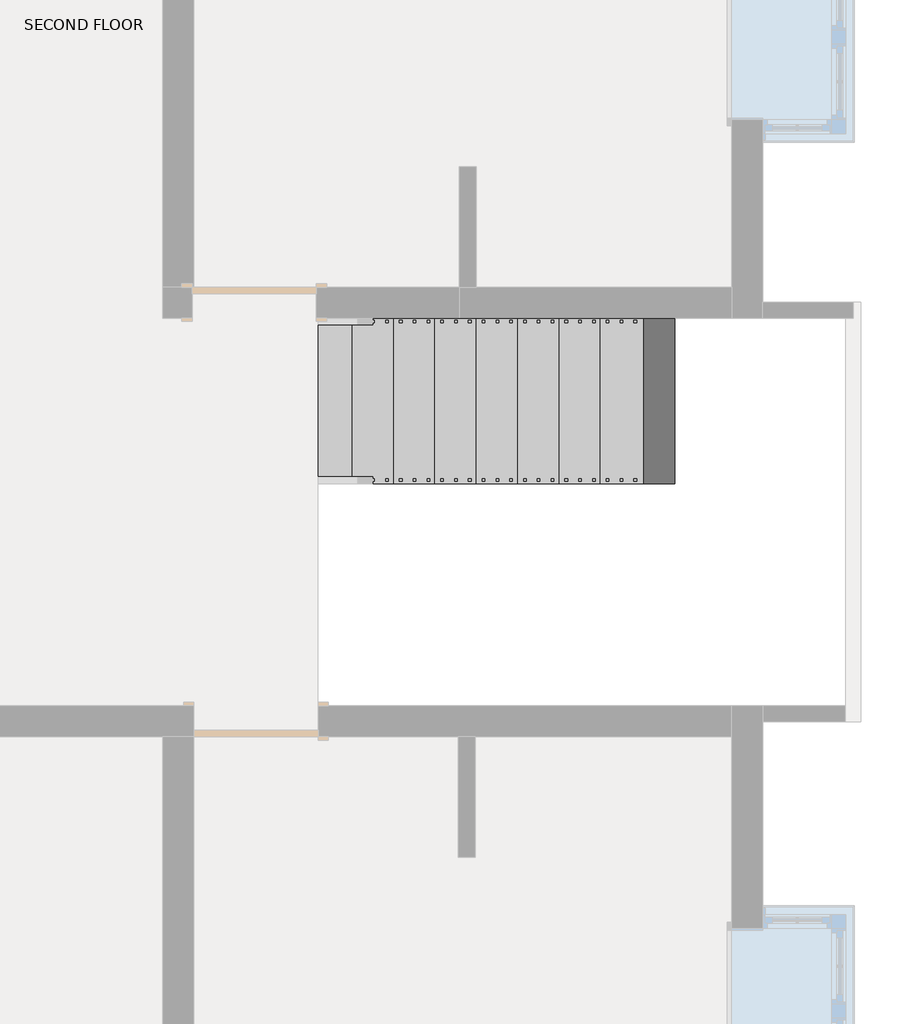
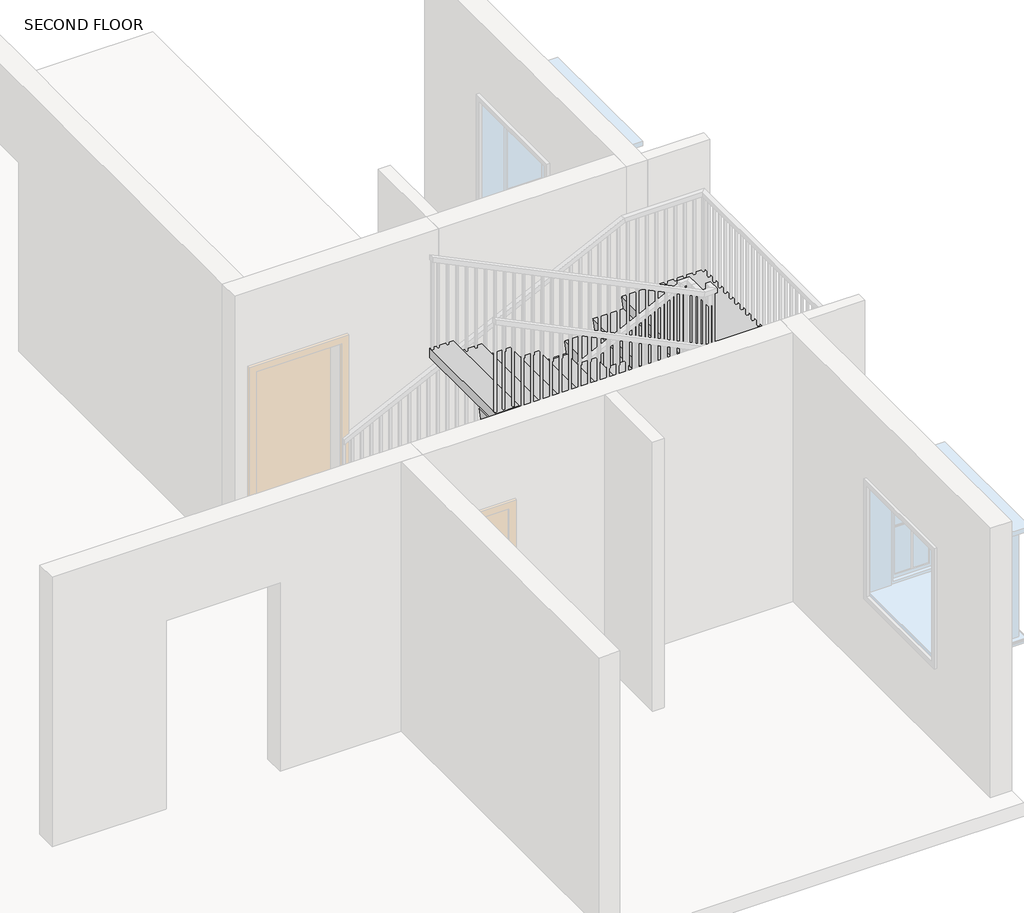
# One storey, part 3 of 6: 1 railing, 1 stair flight.
"""IFC4 building model written with IfcOpenShell, lengths in millimetres."""

from ifc_helpers import new_model, si_unit, frame, origin, place, context, project, spatial, polyline, outline, extrude, faceted_brep, element, save

model = new_model("IFC4")

# Units and contexts
model_context = context("Model", 3, world=origin())
ifc_project = project(units=[si_unit("LENGTHUNIT", "METRE", prefix="MILLI")], contexts=[model_context])

# Site, building, storey
site = spatial("IfcSite", under=ifc_project)
building = spatial("IfcBuilding", under=site)
storey = spatial("IfcBuildingStorey", under=building, Name="SECOND FLOOR", Elevation=6400.8)

# Railing
placement = place(None, origin())
element("IfcRailing", 1, ObjectType="Handrail - Rectangular", at=placement, inside=storey, context=model_context, shape_type="SolidModel", body=[
    faceted_brep([(3126.2584916, -947.666654, 7460.6727273), (3126.2584916, -947.666654, 7404.1956113), (3126.2584916, -998.466654, 7404.1956113), (3126.2584916, -998.466654, 7460.6727273), (6044.5829507, -947.666654, 8878.3823634), (6095.3829507, -947.666654, 8846.5836718), (6095.3829507, -998.466654, 8846.5836718), (6044.5829507, -998.466654, 8878.3823634), (6044.5829507, -947.666654, 8915.4), (6095.3829507, -947.666654, 8864.6), (6095.3829507, -998.466654, 8864.6), (6044.5829507, -998.466654, 8915.4), (6171.5829507, -947.666654, 8915.4), (6171.5829507, -947.666654, 8864.6), (6120.7829507, -998.466654, 8864.6), (6120.7829507, -998.466654, 8915.4), (6171.5829507, -1074.666654, 8915.4), (6171.5829507, -1074.666654, 8864.6), (6120.7829507, -1074.666654, 8864.6), (6120.7829507, -1074.666654, 8915.4), (6171.5829507, -1341.366654, 8915.4), (6171.5829507, -1392.166654, 8864.6), (6120.7829507, -1392.166654, 8864.6), (6120.7829507, -1341.366654, 8915.4), (6171.5829507, -1341.366654, 9097.8903639), (6171.5829507, -1392.166654, 9047.0903639), (6120.7829507, -1392.166654, 9047.0903639), (6120.7829507, -1341.366654, 9097.8903639), (6171.5829507, -1468.366654, 9097.8903639), (6171.5829507, -1468.366654, 9047.0903639), (6120.7829507, -1417.566654, 9047.0903639), (6120.7829507, -1417.566654, 9097.8903639), (6044.5829507, -1468.366654, 9097.8903639), (6032.8967309, -1468.366654, 9047.0903639), (6032.8967309, -1417.566654, 9047.0903639), (6044.5829507, -1417.566654, 9097.8903639), (3126.2584916, -1468.366654, 10515.6), (3126.2584916, -1417.566654, 10515.6), (3126.2584916, -1417.566654, 10459.122884), (3126.2584916, -1468.366654, 10459.122884)], [[[0, 1, 2, 3]], [[1, 0, 4, 5]], [[2, 1, 5, 6]], [[3, 2, 6, 7]], [[0, 3, 7, 4]], [[5, 4, 8, 9]], [[6, 5, 9, 10]], [[7, 6, 10, 11]], [[4, 7, 11, 8]], [[9, 8, 12, 13]], [[10, 9, 13, 14]], [[11, 10, 14, 15]], [[8, 11, 15, 12]], [[13, 12, 16, 17]], [[14, 13, 17, 18]], [[15, 14, 18, 19]], [[12, 15, 19, 16]], [[17, 16, 20, 21]], [[18, 17, 21, 22]], [[19, 18, 22, 23]], [[16, 19, 23, 20]], [[21, 20, 24, 25]], [[22, 21, 25, 26]], [[23, 22, 26, 27]], [[20, 23, 27, 24]], [[25, 24, 28, 29]], [[26, 25, 29, 30]], [[27, 26, 30, 31]], [[24, 27, 31, 28]], [[29, 28, 32, 33]], [[30, 29, 33, 34]], [[31, 30, 34, 35]], [[28, 31, 35, 32]], [[36, 37, 38, 39]], [[33, 32, 36, 39]], [[34, 33, 39, 38]], [[35, 34, 38, 37]], [[32, 35, 37, 36]]]),
    extrude(outline(polyline([(10418.7778093, 3209.3079507), (10428.0322184, 3190.2579507), (9455.7272727, 3190.2579507), (9455.7272727, 3209.3079507), (10418.7778093, 3209.3079507)])), frame((0.0, -1452.491654, 0.0), z_axis=(0.0, 1.0, 0.0), x_axis=(0.0, 0.0, 1.0)), (0.0, 0.0, 1.0), 19.05),
    extrude(outline(polyline([(10369.4209605, 3310.9079507), (10378.6753696, 3291.8579507), (9455.7272727, 3291.8579507), (9455.7272727, 3310.9079507), (10369.4209605, 3310.9079507)])), frame((0.0, -1452.491654, 0.0), z_axis=(0.0, 1.0, 0.0), x_axis=(0.0, 0.0, 1.0)), (0.0, 0.0, 1.0), 19.05),
    extrude(outline(polyline([(10320.0641117, 3412.5079507), (10329.3185208, 3393.4579507), (9310.2545455, 3393.4579507), (9310.2545455, 3412.5079507), (10320.0641117, 3412.5079507)])), frame((0.0, -1452.491654, 0.0), z_axis=(0.0, 1.0, 0.0), x_axis=(0.0, 0.0, 1.0)), (0.0, 0.0, 1.0), 19.05),
    extrude(outline(polyline([(10270.7072629, 3514.1079507), (10279.9616721, 3495.0579507), (9310.2545455, 3495.0579507), (9310.2545455, 3514.1079507), (10270.7072629, 3514.1079507)])), frame((0.0, -1452.491654, 0.0), z_axis=(0.0, 1.0, 0.0), x_axis=(0.0, 0.0, 1.0)), (0.0, 0.0, 1.0), 19.05),
    extrude(outline(polyline([(10221.3504141, 3615.7079507), (10230.6048233, 3596.6579507), (9310.2545455, 3596.6579507), (9310.2545455, 3615.7079507), (10221.3504141, 3615.7079507)])), frame((0.0, -1452.491654, 0.0), z_axis=(0.0, 1.0, 0.0), x_axis=(0.0, 0.0, 1.0)), (0.0, 0.0, 1.0), 19.05),
    extrude(outline(polyline([(10171.9935653, 3717.3079507), (10181.2479745, 3698.2579507), (9164.7818182, 3698.2579507), (9164.7818182, 3717.3079507), (10171.9935653, 3717.3079507)])), frame((0.0, -1452.491654, 0.0), z_axis=(0.0, 1.0, 0.0), x_axis=(0.0, 0.0, 1.0)), (0.0, 0.0, 1.0), 19.05),
    extrude(outline(polyline([(10122.6367166, 3818.9079507), (10131.8911257, 3799.8579507), (9164.7818182, 3799.8579507), (9164.7818182, 3818.9079507), (10122.6367166, 3818.9079507)])), frame((0.0, -1452.491654, 0.0), z_axis=(0.0, 1.0, 0.0), x_axis=(0.0, 0.0, 1.0)), (0.0, 0.0, 1.0), 19.05),
    extrude(outline(polyline([(10073.2798678, 3920.5079507), (10082.5342769, 3901.4579507), (9164.7818182, 3901.4579507), (9164.7818182, 3920.5079507), (10073.2798678, 3920.5079507)])), frame((0.0, -1452.491654, 0.0), z_axis=(0.0, 1.0, 0.0), x_axis=(0.0, 0.0, 1.0)), (0.0, 0.0, 1.0), 19.05),
    extrude(outline(polyline([(10023.923019, 4022.1079507), (10033.1774281, 4003.0579507), (9019.3090909, 4003.0579507), (9019.3090909, 4022.1079507), (10023.923019, 4022.1079507)])), frame((0.0, -1452.491654, 0.0), z_axis=(0.0, 1.0, 0.0), x_axis=(0.0, 0.0, 1.0)), (0.0, 0.0, 1.0), 19.05),
    extrude(outline(polyline([(9974.5661702, 4123.7079507), (9983.8205793, 4104.6579507), (9019.3090909, 4104.6579507), (9019.3090909, 4123.7079507), (9974.5661702, 4123.7079507)])), frame((0.0, -1452.491654, 0.0), z_axis=(0.0, 1.0, 0.0), x_axis=(0.0, 0.0, 1.0)), (0.0, 0.0, 1.0), 19.05),
    extrude(outline(polyline([(9925.2093214, 4225.3079507), (9934.4637306, 4206.2579507), (9019.3090909, 4206.2579507), (9019.3090909, 4225.3079507), (9925.2093214, 4225.3079507)])), frame((0.0, -1452.491654, 0.0), z_axis=(0.0, 1.0, 0.0), x_axis=(0.0, 0.0, 1.0)), (0.0, 0.0, 1.0), 19.05),
    extrude(outline(polyline([(9875.8524726, 4326.9079507), (9885.1068818, 4307.8579507), (8873.8363636, 4307.8579507), (8873.8363636, 4326.9079507), (9875.8524726, 4326.9079507)])), frame((0.0, -1452.491654, 0.0), z_axis=(0.0, 1.0, 0.0), x_axis=(0.0, 0.0, 1.0)), (0.0, 0.0, 1.0), 19.05),
    extrude(outline(polyline([(9826.4956238, 4428.5079507), (9835.750033, 4409.4579507), (8873.8363636, 4409.4579507), (8873.8363636, 4428.5079507), (9826.4956238, 4428.5079507)])), frame((0.0, -1452.491654, 0.0), z_axis=(0.0, 1.0, 0.0), x_axis=(0.0, 0.0, 1.0)), (0.0, 0.0, 1.0), 19.05),
    extrude(outline(polyline([(9777.1387751, 4530.1079507), (9786.3931842, 4511.0579507), (8873.8363636, 4511.0579507), (8873.8363636, 4530.1079507), (9777.1387751, 4530.1079507)])), frame((0.0, -1452.491654, 0.0), z_axis=(0.0, 1.0, 0.0), x_axis=(0.0, 0.0, 1.0)), (0.0, 0.0, 1.0), 19.05),
    extrude(outline(polyline([(9727.7819263, 4631.7079507), (9737.0363354, 4612.6579507), (8728.3636364, 4612.6579507), (8728.3636364, 4631.7079507), (9727.7819263, 4631.7079507)])), frame((0.0, -1452.491654, 0.0), z_axis=(0.0, 1.0, 0.0), x_axis=(0.0, 0.0, 1.0)), (0.0, 0.0, 1.0), 19.05),
    extrude(outline(polyline([(9678.4250775, 4733.3079507), (9687.6794866, 4714.2579507), (8728.3636364, 4714.2579507), (8728.3636364, 4733.3079507), (9678.4250775, 4733.3079507)])), frame((0.0, -1452.491654, 0.0), z_axis=(0.0, 1.0, 0.0), x_axis=(0.0, 0.0, 1.0)), (0.0, 0.0, 1.0), 19.05),
    extrude(outline(polyline([(9629.0682287, 4834.9079507), (9638.3226379, 4815.8579507), (8728.3636364, 4815.8579507), (8728.3636364, 4834.9079507), (9629.0682287, 4834.9079507)])), frame((0.0, -1452.491654, 0.0), z_axis=(0.0, 1.0, 0.0), x_axis=(0.0, 0.0, 1.0)), (0.0, 0.0, 1.0), 19.05),
    extrude(outline(polyline([(9579.7113799, 4936.5079507), (9588.9657891, 4917.4579507), (8582.8909091, 4917.4579507), (8582.8909091, 4936.5079507), (9579.7113799, 4936.5079507)])), frame((0.0, -1452.491654, 0.0), z_axis=(0.0, 1.0, 0.0), x_axis=(0.0, 0.0, 1.0)), (0.0, 0.0, 1.0), 19.05),
    extrude(outline(polyline([(9530.3545311, 5038.1079507), (9539.6089403, 5019.0579507), (8582.8909091, 5019.0579507), (8582.8909091, 5038.1079507), (9530.3545311, 5038.1079507)])), frame((0.0, -1452.491654, 0.0), z_axis=(0.0, 1.0, 0.0), x_axis=(0.0, 0.0, 1.0)), (0.0, 0.0, 1.0), 19.05),
    extrude(outline(polyline([(9480.9976824, 5139.7079507), (9490.2520915, 5120.6579507), (8582.8909091, 5120.6579507), (8582.8909091, 5139.7079507), (9480.9976824, 5139.7079507)])), frame((0.0, -1452.491654, 0.0), z_axis=(0.0, 1.0, 0.0), x_axis=(0.0, 0.0, 1.0)), (0.0, 0.0, 1.0), 19.05),
    extrude(outline(polyline([(9431.559384, 5241.3079507), (9440.8137931, 5222.2579507), (8437.4181818, 5222.2579507), (8437.4181818, 5241.3079507), (9431.559384, 5241.3079507)])), frame((0.0, -1452.491654, 0.0), z_axis=(0.0, 1.0, 0.0), x_axis=(0.0, 0.0, 1.0)), (0.0, 0.0, 1.0), 19.05),
    extrude(outline(polyline([(9382.2839848, 5342.9079507), (9391.5383939, 5323.8579507), (8437.4181818, 5323.8579507), (8437.4181818, 5342.9079507), (9382.2839848, 5342.9079507)])), frame((0.0, -1452.491654, 0.0), z_axis=(0.0, 1.0, 0.0), x_axis=(0.0, 0.0, 1.0)), (0.0, 0.0, 1.0), 19.05),
    extrude(outline(polyline([(9332.927136, 5444.5079507), (9342.1815452, 5425.4579507), (8437.4181818, 5425.4579507), (8437.4181818, 5444.5079507), (9332.927136, 5444.5079507)])), frame((0.0, -1452.491654, 0.0), z_axis=(0.0, 1.0, 0.0), x_axis=(0.0, 0.0, 1.0)), (0.0, 0.0, 1.0), 19.05),
    extrude(outline(polyline([(9283.5702872, 5546.1079507), (9292.8246964, 5527.0579507), (8291.9454545, 5527.0579507), (8291.9454545, 5546.1079507), (9283.5702872, 5546.1079507)])), frame((0.0, -1452.491654, 0.0), z_axis=(0.0, 1.0, 0.0), x_axis=(0.0, 0.0, 1.0)), (0.0, 0.0, 1.0), 19.05),
    extrude(outline(polyline([(9234.2134384, 5647.7079507), (9243.4678476, 5628.6579507), (8291.9454545, 5628.6579507), (8291.9454545, 5647.7079507), (9234.2134384, 5647.7079507)])), frame((0.0, -1452.491654, 0.0), z_axis=(0.0, 1.0, 0.0), x_axis=(0.0, 0.0, 1.0)), (0.0, 0.0, 1.0), 19.05),
    extrude(outline(polyline([(9184.8565897, 5749.3079507), (9194.1109988, 5730.2579507), (8291.9454545, 5730.2579507), (8291.9454545, 5749.3079507), (9184.8565897, 5749.3079507)])), frame((0.0, -1452.491654, 0.0), z_axis=(0.0, 1.0, 0.0), x_axis=(0.0, 0.0, 1.0)), (0.0, 0.0, 1.0), 19.05),
    extrude(outline(polyline([(9135.4997409, 5850.9079507), (9144.75415, 5831.8579507), (8146.4727273, 5831.8579507), (8146.4727273, 5850.9079507), (9135.4997409, 5850.9079507)])), frame((0.0, -1452.491654, 0.0), z_axis=(0.0, 1.0, 0.0), x_axis=(0.0, 0.0, 1.0)), (0.0, 0.0, 1.0), 19.05),
    extrude(outline(polyline([(9086.1428921, 5952.5079507), (9095.3973012, 5933.4579507), (8146.4727273, 5933.4579507), (8146.4727273, 5952.5079507), (9086.1428921, 5952.5079507)])), frame((0.0, -1452.491654, 0.0), z_axis=(0.0, 1.0, 0.0), x_axis=(0.0, 0.0, 1.0)), (0.0, 0.0, 1.0), 19.05),
    extrude(outline(polyline([(9036.7860433, 6054.1079507), (9046.0404524, 6035.0579507), (8146.4727273, 6035.0579507), (8146.4727273, 6054.1079507), (9036.7860433, 6054.1079507)])), frame((0.0, -1452.491654, 0.0), z_axis=(0.0, 1.0, 0.0), x_axis=(0.0, 0.0, 1.0)), (0.0, 0.0, 1.0), 19.05),
    extrude(outline(polyline([(6136.6579507, -1369.941654), (6155.7079507, -1369.941654), (6155.7079507, -1388.991654), (6136.6579507, -1388.991654), (6136.6579507, -1369.941654)])), frame((0.0, 0.0, 8001.0), z_axis=(0.0, 0.0, 1.0), x_axis=(1.0, 0.0, 0.0)), (0.0, 0.0, 1.0), 1046.0903639),
    extrude(outline(polyline([(6136.6579507, -1268.341654), (6155.7079507, -1268.341654), (6155.7079507, -1287.391654), (6136.6579507, -1287.391654), (6136.6579507, -1268.341654)])), frame((0.0, 0.0, 8001.0), z_axis=(0.0, 0.0, 1.0), x_axis=(1.0, 0.0, 0.0)), (0.0, 0.0, 1.0), 863.6),
    extrude(outline(polyline([(6136.6579507, -1166.741654), (6155.7079507, -1166.741654), (6155.7079507, -1185.791654), (6136.6579507, -1185.791654), (6136.6579507, -1166.741654)])), frame((0.0, 0.0, 8001.0), z_axis=(0.0, 0.0, 1.0), x_axis=(1.0, 0.0, 0.0)), (0.0, 0.0, 1.0), 863.6),
    extrude(outline(polyline([(6136.6579507, -1065.141654), (6155.7079507, -1065.141654), (6155.7079507, -1084.191654), (6136.6579507, -1084.191654), (6136.6579507, -1065.141654)])), frame((0.0, 0.0, 8001.0), z_axis=(0.0, 0.0, 1.0), x_axis=(1.0, 0.0, 0.0)), (0.0, 0.0, 1.0), 863.6),
    extrude(outline(polyline([(6063.1334916, -982.591654), (6063.1334916, -963.541654), (6082.1834916, -963.541654), (6082.1834916, -982.591654), (6063.1334916, -982.591654)])), frame((0.0, 0.0, 7855.5272727), z_axis=(0.0, 0.0, 1.0), x_axis=(1.0, 0.0, 0.0)), (0.0, 0.0, 1.0), 1009.0727273),
    extrude(outline(polyline([(8790.8145818, 5980.5834916), (8781.5601727, 5961.5334916), (7855.5272727, 5961.5334916), (7855.5272727, 5980.5834916), (8790.8145818, 5980.5834916)])), frame((0.0, -982.591654, 0.0), z_axis=(0.0, 1.0, 0.0), x_axis=(0.0, 0.0, 1.0)), (0.0, 0.0, 1.0), 19.05),
    extrude(outline(polyline([(8741.457733, 5878.9834916), (8732.2033239, 5859.9334916), (7855.5272727, 5859.9334916), (7855.5272727, 5878.9834916), (8741.457733, 5878.9834916)])), frame((0.0, -982.591654, 0.0), z_axis=(0.0, 1.0, 0.0), x_axis=(0.0, 0.0, 1.0)), (0.0, 0.0, 1.0), 19.05),
    extrude(outline(polyline([(8692.1008843, 5777.3834916), (8682.8464751, 5758.3334916), (7710.0545455, 5758.3334916), (7710.0545455, 5777.3834916), (8692.1008843, 5777.3834916)])), frame((0.0, -982.591654, 0.0), z_axis=(0.0, 1.0, 0.0), x_axis=(0.0, 0.0, 1.0)), (0.0, 0.0, 1.0), 19.05),
    extrude(outline(polyline([(8642.7440355, 5675.7834916), (8633.4896263, 5656.7334916), (7710.0545455, 5656.7334916), (7710.0545455, 5675.7834916), (8642.7440355, 5675.7834916)])), frame((0.0, -982.591654, 0.0), z_axis=(0.0, 1.0, 0.0), x_axis=(0.0, 0.0, 1.0)), (0.0, 0.0, 1.0), 19.05),
    extrude(outline(polyline([(8593.3871867, 5574.1834916), (8584.1327775, 5555.1334916), (7710.0545455, 5555.1334916), (7710.0545455, 5574.1834916), (8593.3871867, 5574.1834916)])), frame((0.0, -982.591654, 0.0), z_axis=(0.0, 1.0, 0.0), x_axis=(0.0, 0.0, 1.0)), (0.0, 0.0, 1.0), 19.05),
    extrude(outline(polyline([(8544.0303379, 5472.5834916), (8534.7759288, 5453.5334916), (7564.5818182, 5453.5334916), (7564.5818182, 5472.5834916), (8544.0303379, 5472.5834916)])), frame((0.0, -982.591654, 0.0), z_axis=(0.0, 1.0, 0.0), x_axis=(0.0, 0.0, 1.0)), (0.0, 0.0, 1.0), 19.05),
    extrude(outline(polyline([(8494.6734891, 5370.9834916), (8485.41908, 5351.9334916), (7564.5818182, 5351.9334916), (7564.5818182, 5370.9834916), (8494.6734891, 5370.9834916)])), frame((0.0, -982.591654, 0.0), z_axis=(0.0, 1.0, 0.0), x_axis=(0.0, 0.0, 1.0)), (0.0, 0.0, 1.0), 19.05),
    extrude(outline(polyline([(8445.3166403, 5269.3834916), (8436.0622312, 5250.3334916), (7564.5818182, 5250.3334916), (7564.5818182, 5269.3834916), (8445.3166403, 5269.3834916)])), frame((0.0, -982.591654, 0.0), z_axis=(0.0, 1.0, 0.0), x_axis=(0.0, 0.0, 1.0)), (0.0, 0.0, 1.0), 19.05),
    extrude(outline(polyline([(8395.9597915, 5167.7834916), (8386.7053824, 5148.7334916), (7419.1090909, 5148.7334916), (7419.1090909, 5167.7834916), (8395.9597915, 5167.7834916)])), frame((0.0, -982.591654, 0.0), z_axis=(0.0, 1.0, 0.0), x_axis=(0.0, 0.0, 1.0)), (0.0, 0.0, 1.0), 19.05),
    extrude(outline(polyline([(8346.6029428, 5066.1834916), (8337.3485336, 5047.1334916), (7419.1090909, 5047.1334916), (7419.1090909, 5066.1834916), (8346.6029428, 5066.1834916)])), frame((0.0, -982.591654, 0.0), z_axis=(0.0, 1.0, 0.0), x_axis=(0.0, 0.0, 1.0)), (0.0, 0.0, 1.0), 19.05),
    extrude(outline(polyline([(8297.246094, 4964.5834916), (8287.9916848, 4945.5334916), (7419.1090909, 4945.5334916), (7419.1090909, 4964.5834916), (8297.246094, 4964.5834916)])), frame((0.0, -982.591654, 0.0), z_axis=(0.0, 1.0, 0.0), x_axis=(0.0, 0.0, 1.0)), (0.0, 0.0, 1.0), 19.05),
    extrude(outline(polyline([(8247.8892452, 4862.9834916), (8238.634836, 4843.9334916), (7273.6363636, 4843.9334916), (7273.6363636, 4862.9834916), (8247.8892452, 4862.9834916)])), frame((0.0, -982.591654, 0.0), z_axis=(0.0, 1.0, 0.0), x_axis=(0.0, 0.0, 1.0)), (0.0, 0.0, 1.0), 19.05),
    extrude(outline(polyline([(8198.5323964, 4761.3834916), (8189.2779873, 4742.3334916), (7273.6363636, 4742.3334916), (7273.6363636, 4761.3834916), (8198.5323964, 4761.3834916)])), frame((0.0, -982.591654, 0.0), z_axis=(0.0, 1.0, 0.0), x_axis=(0.0, 0.0, 1.0)), (0.0, 0.0, 1.0), 19.05),
    extrude(outline(polyline([(8149.1755476, 4659.7834916), (8139.9211385, 4640.7334916), (7273.6363636, 4640.7334916), (7273.6363636, 4659.7834916), (8149.1755476, 4659.7834916)])), frame((0.0, -982.591654, 0.0), z_axis=(0.0, 1.0, 0.0), x_axis=(0.0, 0.0, 1.0)), (0.0, 0.0, 1.0), 19.05),
    extrude(outline(polyline([(8099.8186988, 4558.1834916), (8090.5642897, 4539.1334916), (7128.1636364, 4539.1334916), (7128.1636364, 4558.1834916), (8099.8186988, 4558.1834916)])), frame((0.0, -982.591654, 0.0), z_axis=(0.0, 1.0, 0.0), x_axis=(0.0, 0.0, 1.0)), (0.0, 0.0, 1.0), 19.05),
    extrude(outline(polyline([(8050.4618501, 4456.5834916), (8041.2074409, 4437.5334916), (7128.1636364, 4437.5334916), (7128.1636364, 4456.5834916), (8050.4618501, 4456.5834916)])), frame((0.0, -982.591654, 0.0), z_axis=(0.0, 1.0, 0.0), x_axis=(0.0, 0.0, 1.0)), (0.0, 0.0, 1.0), 19.05),
    extrude(outline(polyline([(8001.1050013, 4354.9834916), (7991.8505921, 4335.9334916), (7128.1636364, 4335.9334916), (7128.1636364, 4354.9834916), (8001.1050013, 4354.9834916)])), frame((0.0, -982.591654, 0.0), z_axis=(0.0, 1.0, 0.0), x_axis=(0.0, 0.0, 1.0)), (0.0, 0.0, 1.0), 19.05),
    extrude(outline(polyline([(7951.7481525, 4253.3834916), (7942.4937433, 4234.3334916), (6982.6909091, 4234.3334916), (6982.6909091, 4253.3834916), (7951.7481525, 4253.3834916)])), frame((0.0, -982.591654, 0.0), z_axis=(0.0, 1.0, 0.0), x_axis=(0.0, 0.0, 1.0)), (0.0, 0.0, 1.0), 19.05),
    extrude(outline(polyline([(7902.3913037, 4151.7834916), (7893.1368946, 4132.7334916), (6982.6909091, 4132.7334916), (6982.6909091, 4151.7834916), (7902.3913037, 4151.7834916)])), frame((0.0, -982.591654, 0.0), z_axis=(0.0, 1.0, 0.0), x_axis=(0.0, 0.0, 1.0)), (0.0, 0.0, 1.0), 19.05),
    extrude(outline(polyline([(7853.0344549, 4050.1834916), (7843.7800458, 4031.1334916), (6982.6909091, 4031.1334916), (6982.6909091, 4050.1834916), (7853.0344549, 4050.1834916)])), frame((0.0, -982.591654, 0.0), z_axis=(0.0, 1.0, 0.0), x_axis=(0.0, 0.0, 1.0)), (0.0, 0.0, 1.0), 19.05),
    extrude(outline(polyline([(7803.6776061, 3948.5834916), (7794.423197, 3929.5334916), (6837.2181818, 3929.5334916), (6837.2181818, 3948.5834916), (7803.6776061, 3948.5834916)])), frame((0.0, -982.591654, 0.0), z_axis=(0.0, 1.0, 0.0), x_axis=(0.0, 0.0, 1.0)), (0.0, 0.0, 1.0), 19.05),
    extrude(outline(polyline([(7754.3207573, 3846.9834916), (7745.0663482, 3827.9334916), (6837.2181818, 3827.9334916), (6837.2181818, 3846.9834916), (7754.3207573, 3846.9834916)])), frame((0.0, -982.591654, 0.0), z_axis=(0.0, 1.0, 0.0), x_axis=(0.0, 0.0, 1.0)), (0.0, 0.0, 1.0), 19.05),
    extrude(outline(polyline([(7704.9639086, 3745.3834916), (7695.7094994, 3726.3334916), (6837.2181818, 3726.3334916), (6837.2181818, 3745.3834916), (7704.9639086, 3745.3834916)])), frame((0.0, -982.591654, 0.0), z_axis=(0.0, 1.0, 0.0), x_axis=(0.0, 0.0, 1.0)), (0.0, 0.0, 1.0), 19.05),
    extrude(outline(polyline([(7655.6070598, 3643.7834916), (7646.3526506, 3624.7334916), (6691.7454545, 3624.7334916), (6691.7454545, 3643.7834916), (7655.6070598, 3643.7834916)])), frame((0.0, -982.591654, 0.0), z_axis=(0.0, 1.0, 0.0), x_axis=(0.0, 0.0, 1.0)), (0.0, 0.0, 1.0), 19.05),
    extrude(outline(polyline([(7606.250211, 3542.1834916), (7596.9958018, 3523.1334916), (6691.7454545, 3523.1334916), (6691.7454545, 3542.1834916), (7606.250211, 3542.1834916)])), frame((0.0, -982.591654, 0.0), z_axis=(0.0, 1.0, 0.0), x_axis=(0.0, 0.0, 1.0)), (0.0, 0.0, 1.0), 19.05),
    extrude(outline(polyline([(7556.8933622, 3440.5834916), (7547.6389531, 3421.5334916), (6691.7454545, 3421.5334916), (6691.7454545, 3440.5834916), (7556.8933622, 3440.5834916)])), frame((0.0, -982.591654, 0.0), z_axis=(0.0, 1.0, 0.0), x_axis=(0.0, 0.0, 1.0)), (0.0, 0.0, 1.0), 19.05),
    extrude(outline(polyline([(7507.5365134, 3338.9834916), (7498.2821043, 3319.9334916), (6546.2727273, 3319.9334916), (6546.2727273, 3338.9834916), (7507.5365134, 3338.9834916)])), frame((0.0, -982.591654, 0.0), z_axis=(0.0, 1.0, 0.0), x_axis=(0.0, 0.0, 1.0)), (0.0, 0.0, 1.0), 19.05),
    extrude(outline(polyline([(7458.1796646, 3237.3834916), (7448.9252555, 3218.3334916), (6546.2727273, 3218.3334916), (6546.2727273, 3237.3834916), (7458.1796646, 3237.3834916)])), frame((0.0, -982.591654, 0.0), z_axis=(0.0, 1.0, 0.0), x_axis=(0.0, 0.0, 1.0)), (0.0, 0.0, 1.0), 19.05),
    extrude(outline(polyline([(6136.6579507, -1433.441654), (6155.7079507, -1433.441654), (6155.7079507, -1452.491654), (6136.6579507, -1452.491654), (6136.6579507, -1433.441654)])), frame((0.0, 0.0, 8001.0), z_axis=(0.0, 0.0, 1.0), x_axis=(1.0, 0.0, 0.0)), (0.0, 0.0, 1.0), 1046.0903639),
    extrude(outline(polyline([(6136.6579507, -982.591654), (6136.6579507, -963.541654), (6155.7079507, -963.541654), (6155.7079507, -982.591654), (6136.6579507, -982.591654)])), frame((0.0, 0.0, 8001.0), z_axis=(0.0, 0.0, 1.0), x_axis=(1.0, 0.0, 0.0)), (0.0, 0.0, 1.0), 863.6),
    extrude(outline(polyline([(10449.8684749, 3145.3084916), (10459.122884, 3126.2584916), (9455.7272727, 3126.2584916), (9455.7272727, 3145.3084916), (10449.8684749, 3145.3084916)])), frame((0.0, -1452.491654, 0.0), z_axis=(0.0, 1.0, 0.0), x_axis=(0.0, 0.0, 1.0)), (0.0, 0.0, 1.0), 19.05),
    extrude(outline(polyline([(7413.4500204, 3145.3084916), (7404.1956113, 3126.2584916), (6546.2727273, 3126.2584916), (6546.2727273, 3145.3084916), (7413.4500204, 3145.3084916)])), frame((0.0, -982.591654, 0.0), z_axis=(0.0, 1.0, 0.0), x_axis=(0.0, 0.0, 1.0)), (0.0, 0.0, 1.0), 19.05),
])

# Stair flight
element("IfcStairFlight", 2, ObjectType="3/4\" Nosing", at=placement, inside=storey, context=model_context, shape_type="Brep", body=[
    faceted_brep([(3126.2584916, 220.733346, 6546.2727273), (3126.2584916, -998.466654, 6546.2727273), (3396.6329507, -998.466654, 6546.2727273), (3396.6329507, 220.733346, 6546.2727273), (3396.6329507, 220.733346, 6482.7727273), (3134.5739678, 220.733346, 6482.7727273), (3134.5739678, -998.466654, 6482.7727273), (3396.6329507, -998.466654, 6482.7727273), (3377.5829507, 220.733346, 6691.7454545), (3377.5829507, -998.466654, 6691.7454545), (3411.0096137, -998.466654, 6691.7454545), (3701.4329507, -998.466654, 6691.7454545), (3701.4329507, 220.733346, 6691.7454545), (3411.0096137, 220.733346, 6691.7454545), (3701.4329507, 220.733346, 6621.3838654), (3411.0096137, 220.733346, 6482.7727273), (3411.0096137, -998.466654, 6482.7727273), (3701.4329507, -998.466654, 6621.3838654), (3682.3829507, 220.733346, 6837.2181818), (3682.3829507, -998.466654, 6837.2181818), (4006.2329507, -998.466654, 6837.2181818), (4006.2329507, 220.733346, 6837.2181818), (4006.2329507, 220.733346, 6766.8565927), (4006.2329507, -998.466654, 6766.8565927), (3987.1829507, 220.733346, 6982.6909091), (3987.1829507, -998.466654, 6982.6909091), (4311.0329507, -998.466654, 6982.6909091), (4311.0329507, 220.733346, 6982.6909091), (4311.0329507, 220.733346, 6912.3293199), (4311.0329507, -998.466654, 6912.3293199), (4291.9829507, 220.733346, 7128.1636364), (4291.9829507, -998.466654, 7128.1636364), (4615.8329507, -998.466654, 7128.1636364), (4615.8329507, 220.733346, 7128.1636364), (4615.8329507, 220.733346, 7057.8020472), (4615.8329507, -998.466654, 7057.8020472), (4596.7829507, 220.733346, 7273.6363636), (4596.7829507, -998.466654, 7273.6363636), (4920.6329507, -998.466654, 7273.6363636), (4920.6329507, 220.733346, 7273.6363636), (4920.6329507, 220.733346, 7203.2747745), (4920.6329507, -998.466654, 7203.2747745), (4901.5829507, 220.733346, 7419.1090909), (4901.5829507, -998.466654, 7419.1090909), (5225.4329507, -998.466654, 7419.1090909), (5225.4329507, 220.733346, 7419.1090909), (5225.4329507, 220.733346, 7348.7475018), (5225.4329507, -998.466654, 7348.7475018), (5206.3829507, 220.733346, 7564.5818182), (5206.3829507, -998.466654, 7564.5818182), (5530.2329507, -998.466654, 7564.5818182), (5530.2329507, 220.733346, 7564.5818182), (5530.2329507, 220.733346, 7494.220229), (5530.2329507, -998.466654, 7494.220229), (5511.1829507, 220.733346, 7710.0545455), (5511.1829507, -998.466654, 7710.0545455), (5835.0329507, -998.466654, 7710.0545455), (5835.0329507, 220.733346, 7710.0545455), (5835.0329507, 220.733346, 7639.6929563), (5835.0329507, -998.466654, 7639.6929563), (5815.9829507, 220.733346, 7855.5272727), (5815.9829507, -998.466654, 7855.5272727), (6139.8329507, -998.466654, 7855.5272727), (6139.8329507, 220.733346, 7855.5272727), (6139.8329507, 220.733346, 7785.1656836), (6459.0096137, -998.466654, 7937.5), (6129.0984269, -998.466654, 7937.5), (6101.7329507, -2636.766654, 8001.0), (7009.1350459, -2636.766654, 8001.0), (7009.1350459, 220.733346, 8001.0), (6459.0096137, 220.733346, 8001.0), (6120.7829507, 220.733346, 8001.0), (6120.7829507, -998.466654, 8001.0), (6120.7829507, -1417.566654, 8001.0), (6101.7329507, -1417.566654, 8001.0), (6101.7329507, -2636.766654, 7937.5), (7009.1350459, -2636.766654, 7937.5), (7009.1350459, 220.733346, 7937.5), (6459.0096137, 220.733346, 7937.5), (6120.7829507, -998.466654, 7937.5), (6120.7829507, -1417.566654, 7937.5), (6101.7329507, -1417.566654, 7937.5), (6120.7829507, -2636.766654, 8146.4727273), (6120.7829507, -1417.566654, 8146.4727273), (6087.3562877, -1417.566654, 8146.4727273), (5796.9329507, -1417.566654, 8146.4727273), (5796.9329507, -2636.766654, 8146.4727273), (6087.3562877, -2636.766654, 8146.4727273), (5796.9329507, -2636.766654, 8076.1111381), (6087.3562877, -2636.766654, 7937.5), (6087.3562877, -1417.566654, 7937.5), (5796.9329507, -1417.566654, 8076.1111381), (5815.9829507, -2636.766654, 8291.9454545), (5815.9829507, -1417.566654, 8291.9454545), (5492.1329507, -1417.566654, 8291.9454545), (5492.1329507, -2636.766654, 8291.9454545), (5492.1329507, -2636.766654, 8221.5838654), (5492.1329507, -1417.566654, 8221.5838654), (5511.1829507, -2636.766654, 8437.4181818), (5511.1829507, -1417.566654, 8437.4181818), (5187.3329507, -1417.566654, 8437.4181818), (5187.3329507, -2636.766654, 8437.4181818), (5187.3329507, -2636.766654, 8367.0565927), (5187.3329507, -1417.566654, 8367.0565927), (5206.3829507, -2636.766654, 8582.8909091), (5206.3829507, -1417.566654, 8582.8909091), (4882.5329507, -1417.566654, 8582.8909091), (4882.5329507, -2636.766654, 8582.8909091), (4882.5329507, -2636.766654, 8512.5293199), (4882.5329507, -1417.566654, 8512.5293199), (4901.5829507, -2636.766654, 8728.3636364), (4901.5829507, -1417.566654, 8728.3636364), (4577.7329507, -1417.566654, 8728.3636364), (4577.7329507, -2636.766654, 8728.3636364), (4577.7329507, -2636.766654, 8658.0020472), (4577.7329507, -1417.566654, 8658.0020472), (4596.7829507, -2636.766654, 8873.8363636), (4596.7829507, -1417.566654, 8873.8363636), (4272.9329507, -1417.566654, 8873.8363636), (4272.9329507, -2636.766654, 8873.8363636), (4272.9329507, -2636.766654, 8803.4747745), (4272.9329507, -1417.566654, 8803.4747745), (4291.9829507, -2636.766654, 9019.3090909), (4291.9829507, -1417.566654, 9019.3090909), (3968.1329507, -1417.566654, 9019.3090909), (3968.1329507, -2636.766654, 9019.3090909), (3968.1329507, -2636.766654, 8948.9475018), (3968.1329507, -1417.566654, 8948.9475018), (3987.1829507, -2636.766654, 9164.7818182), (3987.1829507, -1417.566654, 9164.7818182), (3663.3329507, -1417.566654, 9164.7818182), (3663.3329507, -2636.766654, 9164.7818182), (3663.3329507, -2636.766654, 9094.420229), (3663.3329507, -1417.566654, 9094.420229), (3682.3829507, -2636.766654, 9310.2545455), (3682.3829507, -1417.566654, 9310.2545455), (3358.5329507, -1417.566654, 9310.2545455), (3358.5329507, -2636.766654, 9310.2545455), (3358.5329507, -2636.766654, 9239.8929563), (3358.5329507, -1417.566654, 9239.8929563), (3377.5829507, -2636.766654, 9455.7272727), (3377.5829507, -1417.566654, 9455.7272727), (3126.2584916, -1417.566654, 9455.7272727), (3126.2584916, -2636.766654, 9455.7272727), (3126.2584916, -2636.766654, 9350.7512209), (3126.2584916, -1417.566654, 9350.7512209)], [[[0, 1, 2, 3]], [[0, 3, 4, 5]], [[2, 1, 6, 7]], [[8, 9, 10, 11, 12, 13]], [[3, 8, 13, 12, 14, 15, 4]], [[9, 2, 7, 16, 17, 11, 10]], [[18, 19, 20, 21]], [[18, 21, 22, 14, 12]], [[20, 19, 11, 17, 23]], [[24, 25, 26, 27]], [[24, 27, 28, 22, 21]], [[26, 25, 20, 23, 29]], [[30, 31, 32, 33]], [[30, 33, 34, 28, 27]], [[32, 31, 26, 29, 35]], [[36, 37, 38, 39]], [[36, 39, 40, 34, 33]], [[38, 37, 32, 35, 41]], [[42, 43, 44, 45]], [[42, 45, 46, 40, 39]], [[44, 43, 38, 41, 47]], [[48, 49, 50, 51]], [[48, 51, 52, 46, 45]], [[50, 49, 44, 47, 53]], [[54, 55, 56, 57]], [[54, 57, 58, 52, 51]], [[56, 55, 50, 53, 59]], [[60, 61, 62, 63]], [[60, 63, 64, 58, 57]], [[61, 56, 59, 65, 66, 62]], [[67, 68, 69, 70, 71, 72, 73, 74]], [[68, 67, 75, 76]], [[69, 68, 76, 77]], [[63, 71, 70, 69, 77, 78, 64]], [[72, 66, 79]], [[73, 72, 79, 80]], [[74, 73, 80, 81]], [[82, 83, 84, 85, 86, 87]], [[67, 82, 87, 86, 88, 89, 75]], [[83, 74, 81, 90, 91, 85, 84]], [[92, 93, 94, 95]], [[92, 95, 96, 88, 86]], [[94, 93, 85, 91, 97]], [[98, 99, 100, 101]], [[98, 101, 102, 96, 95]], [[100, 99, 94, 97, 103]], [[104, 105, 106, 107]], [[104, 107, 108, 102, 101]], [[106, 105, 100, 103, 109]], [[110, 111, 112, 113]], [[110, 113, 114, 108, 107]], [[112, 111, 106, 109, 115]], [[116, 117, 118, 119]], [[116, 119, 120, 114, 113]], [[118, 117, 112, 115, 121]], [[122, 123, 124, 125]], [[122, 125, 126, 120, 119]], [[124, 123, 118, 121, 127]], [[128, 129, 130, 131]], [[128, 131, 132, 126, 125]], [[130, 129, 124, 127, 133]], [[134, 135, 136, 137]], [[134, 137, 138, 132, 131]], [[136, 135, 130, 133, 139]], [[140, 141, 142, 143]], [[140, 143, 144, 138, 137]], [[142, 141, 136, 139, 145]], [[143, 142, 145, 144]], [[1, 0, 5, 6]], [[3, 2, 9, 8]], [[12, 11, 19, 18]], [[21, 20, 25, 24]], [[27, 26, 31, 30]], [[33, 32, 37, 36]], [[39, 38, 43, 42]], [[45, 44, 49, 48]], [[51, 50, 55, 54]], [[57, 56, 61, 60]], [[63, 62, 66, 72, 71]], [[67, 74, 83, 82]], [[86, 85, 93, 92]], [[95, 94, 99, 98]], [[101, 100, 105, 104]], [[107, 106, 111, 110]], [[113, 112, 117, 116]], [[119, 118, 123, 122]], [[125, 124, 129, 128]], [[131, 130, 135, 134]], [[137, 136, 141, 140]], [[15, 16, 7, 6, 5, 4]], [[16, 15, 14, 22, 28, 34, 40, 46, 52, 58, 64, 78, 65, 59, 53, 47, 41, 35, 29, 23, 17]], [[65, 78, 77, 76, 75, 89, 90, 81, 80, 79, 66]], [[90, 89, 88, 96, 102, 108, 114, 120, 126, 132, 138, 144, 145, 139, 133, 127, 121, 115, 109, 103, 97, 91]]]),
])

save(model, "model.ifc")

# Revit data of these elements
# Type "Handrail - Rectangular"
#   Assembly Code = "C2010400"
#   built-in parameter 1008612 = 0.0416667 (stored number, unit not read)
#   built-in parameter 1008611 = 0.0416667 (stored number, unit not read)
#   built-in parameter 1008609 = 0.333333 (stored number, unit not read)
#   built-in parameter 1008604 = 0.166667 (stored number, unit not read)
#   built-in parameter 1008603 = 0.166667 (stored number, unit not read)
#   Railing Height = 3' - 0"
#   built-in parameter 1008630 = 2
#   built-in parameter 1008610 = 2
#   built-in parameter 1008618 = Baluster - Square : 3/4"
# Element 1 (IfcRailing, "Handrail - Rectangular")
#   Phase Created = New Construction
# Element 2 (IfcStairFlight, "3/4\" Nosing")
#   Phase Created = New Construction
#   Materials on its faces: "Concrete, Cast-in-Place gray"
# Materials
#   "Concrete, Cast-in-Place gray": class "Concrete", colour RGB 192 192 192, transparency 0, Description = "Cast-in-place concrete", Cost = 0
